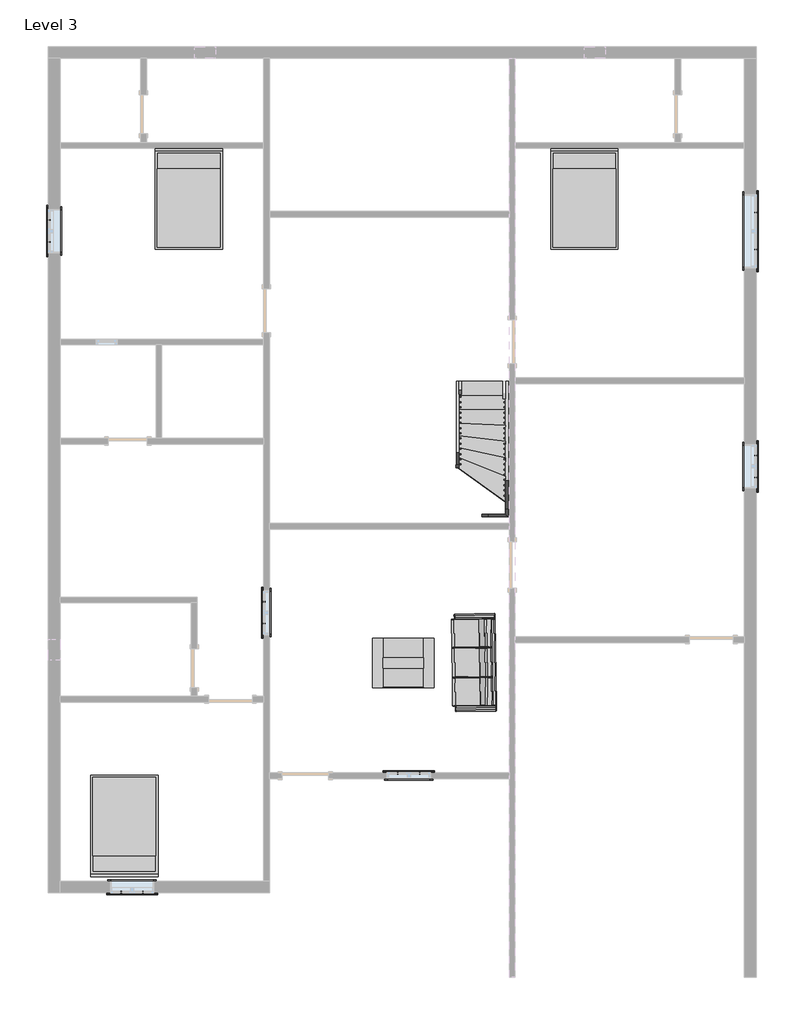
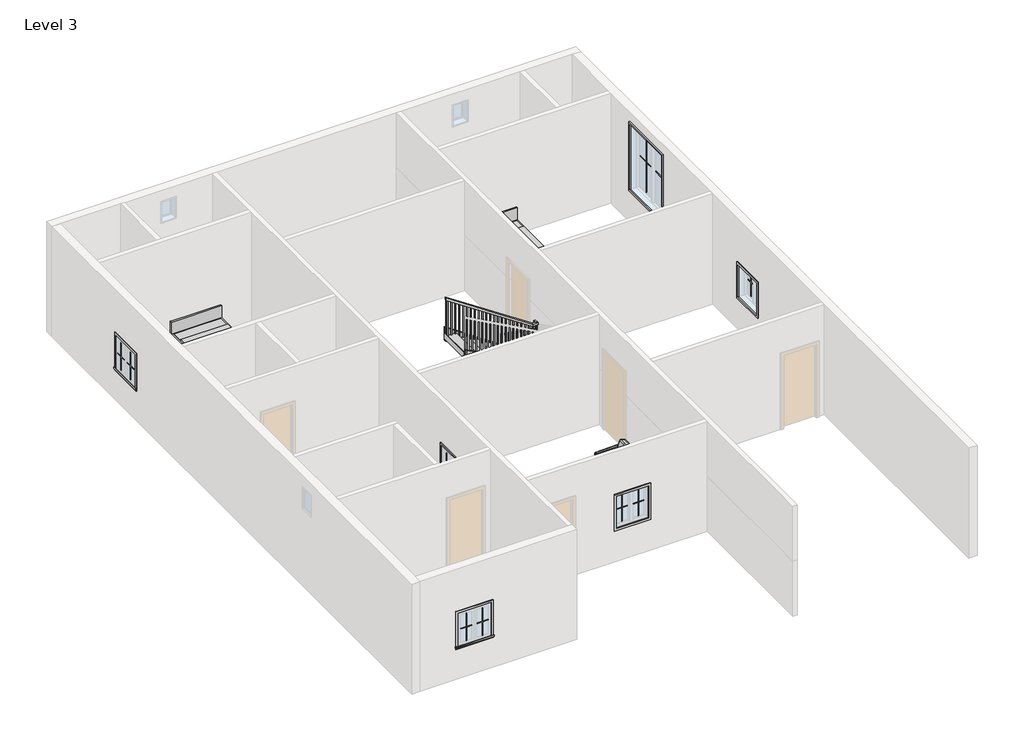
# One storey, part 3 of 3: 24 proxies, 6 members, 5 furniture elements, 1 railing, 1 stair flight.
"""IFC4 building model written with IfcOpenShell, lengths in millimetres."""

from ifc_helpers import new_model, si_unit, frame, origin, place, context, project, spatial, polyline, outline, extrude, faceted_brep, transform, mapped, element, save
from components import muntin_pattern_2x2_muntin_pattern_2x2_b3fe6957, muntin_pattern_2x2_muntin_pattern_2x2_3e0ecaf2, muntin_pattern_2x2_muntin_pattern_2x2_bff912c5, muntin_pattern_2x2_muntin_pattern_2x2_c2194282, trim_window_exterior_flat_with_sill_41619996, trim_window_exterior_flat_with_sill_e04b3088, trim_window_interior_flat_picture_frame_51c85655, trim_window_interior_flat_picture_frame_2a7685fe, furniture_2fc85b74, furniture_29a9adb8, furniture_57072a26, bed_17739_bed_17739_15c61121, wood_and_glass_coffee_table_17065_wood_and_glass_coffee_dbc724b2, stair_flight_11d19efb

model = new_model("IFC4")

# Units and contexts
model_context = context("Model", 3, world=origin())
ifc_project = project(units=[si_unit("LENGTHUNIT", "METRE", prefix="MILLI")], contexts=[model_context])

# Site, building, storey
site = spatial("IfcSite", under=ifc_project)
building = spatial("IfcBuilding", under=site)
storey = spatial("IfcBuildingStorey", under=building, Name="Level 3", Elevation=3200.4)

# Proxies
placement = place(None, origin())
muntin_pattern_2x2_muntin_pattern_2x2_shape = muntin_pattern_2x2_muntin_pattern_2x2_b3fe6957(model_context)
element("IfcBuildingElementProxy", 1, Name="Muntin Pattern_2x2 : Muntin Pattern_2x2", ObjectType="Muntin Pattern_2x2 : Muntin Pattern_2x2", at=placement, inside=storey, context=model_context, shape_type="MappedRepresentation", body=[
    mapped(muntin_pattern_2x2_muntin_pattern_2x2_shape, transform((-7494.1165084, 6600.4397623, 4184.65), x_axis=(0.0, 1.0, 0.0), y_axis=(-1.0, 0.0, 0.0), z_axis=(0.0, 0.0, 1.0))),
])
element("IfcBuildingElementProxy", 2, Name="Muntin Pattern_2x2 : Muntin Pattern_2x2", ObjectType="Muntin Pattern_2x2 : Muntin Pattern_2x2", at=placement, inside=storey, context=model_context, shape_type="MappedRepresentation", body=[
    mapped(muntin_pattern_2x2_muntin_pattern_2x2_shape, transform((-5651.0290084, -6136.0727377, 4184.65), x_axis=(-1.0, 0.0, 0.0), y_axis=(0.0, -1.0, 0.0), z_axis=(0.0, 0.0, 1.0))),
])
element("IfcBuildingElementProxy", 3, Name="Muntin Pattern_2x2 : Muntin Pattern_2x2", ObjectType="Muntin Pattern_2x2 : Muntin Pattern_2x2", at=placement, inside=storey, context=model_context, shape_type="MappedRepresentation", body=[
    mapped(muntin_pattern_2x2_muntin_pattern_2x2_shape, transform((-656.7540084, -3805.6227377, 4184.65), x_axis=(1.0, 0.0, 0.0), y_axis=(0.0, 1.0, 0.0), z_axis=(0.0, 0.0, 1.0))),
])
element("IfcBuildingElementProxy", 4, Name="Muntin Pattern_2x2 : Muntin Pattern_2x2", ObjectType="Muntin Pattern_2x2 : Muntin Pattern_2x2", at=placement, inside=storey, context=model_context, shape_type="MappedRepresentation", body=[
    mapped(muntin_pattern_2x2_muntin_pattern_2x2_shape, transform((6355.2334916, 2418.9647623, 4184.65), x_axis=(0.0, -1.0, 0.0), y_axis=(1.0, 0.0, 0.0), z_axis=(0.0, 0.0, 1.0))),
])
element("IfcBuildingElementProxy", 5, Name="Muntin Pattern_2x2 : Muntin Pattern_2x2", ObjectType="Muntin Pattern_2x2 : Muntin Pattern_2x2", at=placement, inside=storey, context=model_context, shape_type="MappedRepresentation", body=[
    mapped(muntin_pattern_2x2_muntin_pattern_2x2_shape, transform((-3277.7165084, -873.5102377, 4184.65), x_axis=(0.0, 1.0, 0.0), y_axis=(-1.0, 0.0, 0.0), z_axis=(0.0, 0.0, 1.0))),
])
muntin_pattern_2x2_muntin_pattern_2x2_2_shape = muntin_pattern_2x2_muntin_pattern_2x2_3e0ecaf2(model_context)
element("IfcBuildingElementProxy", 6, Name="Muntin Pattern_2x2 : Muntin Pattern_2x2", ObjectType="Muntin Pattern_2x2 : Muntin Pattern_2x2", at=placement, inside=storey, context=model_context, shape_type="MappedRepresentation", body=[
    mapped(muntin_pattern_2x2_muntin_pattern_2x2_2_shape, transform((-7494.1165084, 7029.0647623, 4184.65), x_axis=(0.0, -1.0, 0.0), y_axis=(1.0, 0.0, 0.0), z_axis=(0.0, 0.0, 1.0))),
])
element("IfcBuildingElementProxy", 7, Name="Muntin Pattern_2x2 : Muntin Pattern_2x2", ObjectType="Muntin Pattern_2x2 : Muntin Pattern_2x2", at=placement, inside=storey, context=model_context, shape_type="MappedRepresentation", body=[
    mapped(muntin_pattern_2x2_muntin_pattern_2x2_2_shape, transform((-6079.6540084, -6136.0727377, 4184.65), x_axis=(1.0, 0.0, 0.0), y_axis=(0.0, 1.0, 0.0), z_axis=(0.0, 0.0, 1.0))),
])
element("IfcBuildingElementProxy", 8, Name="Muntin Pattern_2x2 : Muntin Pattern_2x2", ObjectType="Muntin Pattern_2x2 : Muntin Pattern_2x2", at=placement, inside=storey, context=model_context, shape_type="MappedRepresentation", body=[
    mapped(muntin_pattern_2x2_muntin_pattern_2x2_2_shape, transform((-228.1290084, -3805.6227377, 4184.65), x_axis=(-1.0, 0.0, 0.0), y_axis=(0.0, -1.0, 0.0), z_axis=(0.0, 0.0, 1.0))),
])
element("IfcBuildingElementProxy", 9, Name="Muntin Pattern_2x2 : Muntin Pattern_2x2", ObjectType="Muntin Pattern_2x2 : Muntin Pattern_2x2", at=placement, inside=storey, context=model_context, shape_type="MappedRepresentation", body=[
    mapped(muntin_pattern_2x2_muntin_pattern_2x2_2_shape, transform((6355.2334916, 1990.3397623, 4184.65), x_axis=(0.0, 1.0, 0.0), y_axis=(-1.0, 0.0, 0.0), z_axis=(0.0, 0.0, 1.0))),
])
element("IfcBuildingElementProxy", 10, Name="Muntin Pattern_2x2 : Muntin Pattern_2x2", ObjectType="Muntin Pattern_2x2 : Muntin Pattern_2x2", at=placement, inside=storey, context=model_context, shape_type="MappedRepresentation", body=[
    mapped(muntin_pattern_2x2_muntin_pattern_2x2_2_shape, transform((-3277.7165084, -444.8852377, 4184.65), x_axis=(0.0, -1.0, 0.0), y_axis=(1.0, 0.0, 0.0), z_axis=(0.0, 0.0, 1.0))),
])
muntin_pattern_2x2_muntin_pattern_2x2_3_shape = muntin_pattern_2x2_muntin_pattern_2x2_bff912c5(model_context)
element("IfcBuildingElementProxy", 11, Name="Muntin Pattern_2x2 : Muntin Pattern_2x2", ObjectType="Muntin Pattern_2x2 : Muntin Pattern_2x2", at=placement, inside=storey, context=model_context, shape_type="MappedRepresentation", body=[
    mapped(muntin_pattern_2x2_muntin_pattern_2x2_3_shape, transform((6355.2334916, 7175.1147623, 4184.65), x_axis=(0.0, -1.0, 0.0), y_axis=(1.0, 0.0, 0.0), z_axis=(0.0, 0.0, 1.0))),
])
muntin_pattern_2x2_muntin_pattern_2x2_4_shape = muntin_pattern_2x2_muntin_pattern_2x2_c2194282(model_context)
element("IfcBuildingElementProxy", 12, Name="Muntin Pattern_2x2 : Muntin Pattern_2x2", ObjectType="Muntin Pattern_2x2 : Muntin Pattern_2x2", at=placement, inside=storey, context=model_context, shape_type="MappedRepresentation", body=[
    mapped(muntin_pattern_2x2_muntin_pattern_2x2_4_shape, transform((6355.2334916, 6454.3897623, 4184.65), x_axis=(0.0, 1.0, 0.0), y_axis=(-1.0, 0.0, 0.0), z_axis=(0.0, 0.0, 1.0))),
])
trim_window_exterior_flat_with_sill_shape = trim_window_exterior_flat_with_sill_41619996(model_context)
element("IfcBuildingElementProxy", 13, Name="Trim-Window-Exterior-Flat : with Sill", ObjectType="Trim-Window-Exterior-Flat : with Sill", at=placement, inside=storey, context=model_context, shape_type="MappedRepresentation", body=[
    mapped(trim_window_exterior_flat_with_sill_shape, transform((-7503.6415084, 6814.7522623, 5029.2), x_axis=(0.0, -1.0, 0.0), y_axis=(0.0, 0.0, 1.0), z_axis=(-1.0, 0.0, 0.0))),
])
element("IfcBuildingElementProxy", 14, Name="Trim-Window-Exterior-Flat : with Sill", ObjectType="Trim-Window-Exterior-Flat : with Sill", at=placement, inside=storey, context=model_context, shape_type="MappedRepresentation", body=[
    mapped(trim_window_exterior_flat_with_sill_shape, transform((-5865.3415084, -6145.5977377, 5029.2), x_axis=(1.0, 0.0, 0.0), y_axis=(0.0, 0.0, 1.0), z_axis=(0.0, -1.0, 0.0))),
])
element("IfcBuildingElementProxy", 15, Name="Trim-Window-Exterior-Flat : with Sill", ObjectType="Trim-Window-Exterior-Flat : with Sill", at=placement, inside=storey, context=model_context, shape_type="MappedRepresentation", body=[
    mapped(trim_window_exterior_flat_with_sill_shape, transform((-442.4415084, -3796.0977377, 5029.2), x_axis=(-1.0, 0.0, 0.0), y_axis=(0.0, 0.0, 1.0), z_axis=(0.0, 1.0, 0.0))),
])
element("IfcBuildingElementProxy", 16, Name="Trim-Window-Exterior-Flat : with Sill", ObjectType="Trim-Window-Exterior-Flat : with Sill", at=placement, inside=storey, context=model_context, shape_type="MappedRepresentation", body=[
    mapped(trim_window_exterior_flat_with_sill_shape, transform((6364.7584916, 2204.6522623, 5029.2), x_axis=(0.0, 1.0, 0.0), y_axis=(0.0, 0.0, 1.0), z_axis=(1.0, 0.0, 0.0))),
])
element("IfcBuildingElementProxy", 17, Name="Trim-Window-Exterior-Flat : with Sill", ObjectType="Trim-Window-Exterior-Flat : with Sill", at=placement, inside=storey, context=model_context, shape_type="MappedRepresentation", body=[
    mapped(trim_window_exterior_flat_with_sill_shape, transform((-3287.2415084, -659.1977377, 5029.2), x_axis=(0.0, -1.0, 0.0), y_axis=(0.0, 0.0, 1.0), z_axis=(-1.0, 0.0, 0.0))),
])
trim_window_exterior_flat_with_sill_2_shape = trim_window_exterior_flat_with_sill_e04b3088(model_context)
element("IfcBuildingElementProxy", 18, Name="Trim-Window-Exterior-Flat : with Sill", ObjectType="Trim-Window-Exterior-Flat : with Sill", at=placement, inside=storey, context=model_context, shape_type="MappedRepresentation", body=[
    mapped(trim_window_exterior_flat_with_sill_2_shape, transform((6364.7584916, 6814.7522623, 5943.6), x_axis=(0.0, 1.0, 0.0), y_axis=(0.0, 0.0, 1.0), z_axis=(1.0, 0.0, 0.0))),
])
trim_window_interior_flat_picture_frame_shape = trim_window_interior_flat_picture_frame_51c85655(model_context)
element("IfcBuildingElementProxy", 19, Name="Trim-Window-Interior-Flat : Picture Frame", ObjectType="Trim-Window-Interior-Flat : Picture Frame", at=placement, inside=storey, context=model_context, shape_type="MappedRepresentation", body=[
    mapped(trim_window_interior_flat_picture_frame_shape, transform((-7275.0415084, 6814.7522623, 5029.2), x_axis=(0.0, 1.0, 0.0), y_axis=(0.0, 0.0, 1.0), z_axis=(1.0, 0.0, 0.0))),
])
element("IfcBuildingElementProxy", 20, Name="Trim-Window-Interior-Flat : Picture Frame", ObjectType="Trim-Window-Interior-Flat : Picture Frame", at=placement, inside=storey, context=model_context, shape_type="MappedRepresentation", body=[
    mapped(trim_window_interior_flat_picture_frame_shape, transform((-5865.3415084, -5916.9977377, 5029.2), x_axis=(-1.0, 0.0, 0.0), y_axis=(0.0, 0.0, 1.0), z_axis=(0.0, 1.0, 0.0))),
])
element("IfcBuildingElementProxy", 21, Name="Trim-Window-Interior-Flat : Picture Frame", ObjectType="Trim-Window-Interior-Flat : Picture Frame", at=placement, inside=storey, context=model_context, shape_type="MappedRepresentation", body=[
    mapped(trim_window_interior_flat_picture_frame_shape, transform((-442.4415084, -3910.3977377, 5029.2), x_axis=(1.0, 0.0, 0.0), y_axis=(0.0, 0.0, 1.0), z_axis=(0.0, -1.0, 0.0))),
])
element("IfcBuildingElementProxy", 22, Name="Trim-Window-Interior-Flat : Picture Frame", ObjectType="Trim-Window-Interior-Flat : Picture Frame", at=placement, inside=storey, context=model_context, shape_type="MappedRepresentation", body=[
    mapped(trim_window_interior_flat_picture_frame_shape, transform((6136.1584916, 2204.6522623, 5029.2), x_axis=(0.0, -1.0, 0.0), y_axis=(0.0, 0.0, 1.0), z_axis=(-1.0, 0.0, 0.0))),
])
element("IfcBuildingElementProxy", 23, Name="Trim-Window-Interior-Flat : Picture Frame", ObjectType="Trim-Window-Interior-Flat : Picture Frame", at=placement, inside=storey, context=model_context, shape_type="MappedRepresentation", body=[
    mapped(trim_window_interior_flat_picture_frame_shape, transform((-3172.9415084, -659.1977377, 5029.2), x_axis=(0.0, 1.0, 0.0), y_axis=(0.0, 0.0, 1.0), z_axis=(1.0, 0.0, 0.0))),
])
trim_window_interior_flat_picture_frame_2_shape = trim_window_interior_flat_picture_frame_2a7685fe(model_context)
element("IfcBuildingElementProxy", 24, Name="Trim-Window-Interior-Flat : Picture Frame", ObjectType="Trim-Window-Interior-Flat : Picture Frame", at=placement, inside=storey, context=model_context, shape_type="MappedRepresentation", body=[
    mapped(trim_window_interior_flat_picture_frame_2_shape, transform((6136.1584916, 6814.7522623, 5943.6), x_axis=(0.0, -1.0, 0.0), y_axis=(0.0, 0.0, 1.0), z_axis=(-1.0, 0.0, 0.0))),
])

# Furniture
furniture_shape = furniture_2fc85b74(model_context)
furniture_2_shape = furniture_29a9adb8(model_context)
furniture_3_shape = furniture_57072a26(model_context)
element("IfcFurniture", 25, at=placement, inside=storey, context=model_context, shape_type="MappedRepresentation", body=[
    mapped(furniture_shape, transform((460.7695276, -1640.1238257, 3200.4), x_axis=(0.014042050983927294, -0.9999014055416489, 0.0), y_axis=(0.9999014055416489, 0.014042050983927294, 0.0), z_axis=(0.0, 0.0, 1.0))),
    mapped(furniture_2_shape, transform((460.7695276, -1640.1238257, 3200.4), x_axis=(0.014042050983927294, -0.9999014055416489, 0.0), y_axis=(0.9999014055416489, 0.014042050983927294, 0.0), z_axis=(0.0, 0.0, 1.0))),
    mapped(furniture_3_shape, transform((460.7695276, -1640.1238257, 3200.4), x_axis=(0.014042050983927294, -0.9999014055416489, 0.0), y_axis=(0.9999014055416489, 0.014042050983927294, 0.0), z_axis=(0.0, 0.0, 1.0))),
])
bed_17739_bed_17739_shape = bed_17739_bed_17739_15c61121(model_context)
element("IfcFurniture", 26, ObjectType="Bed_17739 : Bed_17739", at=placement, inside=storey, context=model_context, shape_type="MappedRepresentation", body=[
    mapped(bed_17739_bed_17739_shape, transform((-4754.0915084, 7424.3522623, 3200.4), x_axis=(1.0, 0.0, 0.0), y_axis=(0.0, 1.0, 0.0), z_axis=(0.0, 0.0, 1.0))),
])
element("IfcFurniture", 27, ObjectType="Bed_17739 : Bed_17739", at=placement, inside=storey, context=model_context, shape_type="MappedRepresentation", body=[
    mapped(bed_17739_bed_17739_shape, transform((2998.5366507, 7424.3522623, 3200.4), x_axis=(1.0, 0.0, 0.0), y_axis=(0.0, 1.0, 0.0), z_axis=(0.0, 0.0, 1.0))),
])
element("IfcFurniture", 28, ObjectType="Bed_17739 : Bed_17739", at=placement, inside=storey, context=model_context, shape_type="MappedRepresentation", body=[
    mapped(bed_17739_bed_17739_shape, transform((-6017.7415084, -4812.0977377, 3200.4), x_axis=(-1.0, 0.0, 0.0), y_axis=(0.0, -1.0, 0.0), z_axis=(0.0, 0.0, 1.0))),
])
wood_and_glass_coffee_table_17065_wood_and_glass_coffee_shape = wood_and_glass_coffee_table_17065_wood_and_glass_coffee_dbc724b2(model_context)
element("IfcFurniture", 29, ObjectType="Wood_and_Glass_Coffee_Table_17065 : Wood_and_Glass_Coffee_Table_17065", at=placement, inside=storey, context=model_context, shape_type="MappedRepresentation", body=[
    mapped(wood_and_glass_coffee_table_17065_wood_and_glass_coffee_shape, transform((-550.3915084, -1643.4477377, 3200.4), x_axis=(1.0, 0.0, 0.0), y_axis=(0.0, 1.0, 0.0), z_axis=(0.0, 0.0, 1.0))),
])

# Members
element("IfcMember", 30, ObjectType="Stringer - 2\" Width", at=placement, inside=storey, context=model_context, shape_type="SweptSolid", body=[
    extrude(outline(polyline([(3870.4222402, 3434.0789033), (3870.4222402, 3200.4), (3655.4968958, 3200.4), (1369.1992084, 4333.0067011), (1369.1992084, 4673.1572536), (3870.4222402, 3434.0789033)])), frame((1456.2084916, 0.0, 0.0), z_axis=(1.0, 0.0, 0.0), x_axis=(0.0, 1.0, 0.0)), (0.0, 0.0, 1.0), 50.8),
])
element("IfcMember", 31, ObjectType="Stringer - 2\" Width", at=placement, inside=storey, context=model_context, shape_type="SweptSolid", body=[
    extrude(outline(polyline([(1456.2084916, 1369.1992084), (1507.0084916, 1369.1992084), (1507.0084916, 1218.1652728), (1456.2084916, 1268.9652728), (1456.2084916, 1369.1992084)])), frame((0.0, 0.0, 4333.0067011), z_axis=(0.0, 0.0, 1.0), x_axis=(1.0, 0.0, 0.0)), (0.0, 0.0, 1.0), 340.1505525),
])
element("IfcMember", 32, ObjectType="Stringer - 2\" Width", at=placement, inside=storey, context=model_context, shape_type="SweptSolid", body=[
    extrude(outline(polyline([(1456.2084916, 1268.9652728), (1507.0084916, 1218.1652728), (1113.208453, 1218.1652728), (1113.208453, 1268.9652728), (1456.2084916, 1268.9652728)])), frame((0.0, 0.0, 4333.0067011), z_axis=(0.0, 0.0, 1.0), x_axis=(1.0, 0.0, 0.0)), (0.0, 0.0, 1.0), 340.1505525),
])
element("IfcMember", 33, ObjectType="Stringer - 2\" Width", at=placement, inside=storey, context=model_context, shape_type="SweptSolid", body=[
    extrude(outline(polyline([(3870.4222402, 3390.6545013), (3870.4222402, 3200.4), (3614.0281198, 3200.4), (2234.1652728, 4206.8313584), (2234.1652728, 4584.0921868), (3870.4222402, 3390.6545013)])), frame((491.0084916, 0.0, 0.0), z_axis=(1.0, 0.0, 0.0), x_axis=(0.0, 1.0, 0.0)), (0.0, 0.0, 1.0), 50.8),
])
element("IfcMember", 34, ObjectType="Stringer - 2\" Width", at=placement, inside=storey, context=model_context, shape_type="SweptSolid", body=[
    extrude(outline(polyline([(4358.5835681, 541.8084916), (4726.3965617, 541.8084916), (6317.3897736, -1813.7050583), (5949.57678, -1813.7050583), (4358.5835681, 541.8084916)])), frame((0.0, 2183.3652728, 0.0), z_axis=(0.0, 1.0, 0.0), x_axis=(0.0, 0.0, 1.0)), (0.0, 0.0, 1.0), 50.8),
])
element("IfcMember", 35, ObjectType="Stringer - 2\" Width", at=placement, inside=storey, context=model_context, shape_type="SweptSolid", body=[
    extrude(outline(polyline([(4333.0067011, 1113.208453), (4673.1572536, 1113.208453), (6264.3877281, -1813.7050583), (5924.2371756, -1813.7050583), (4333.0067011, 1113.208453)])), frame((0.0, 1218.1652728, 0.0), z_axis=(0.0, 1.0, 0.0), x_axis=(0.0, 0.0, 1.0)), (0.0, 0.0, 1.0), 50.8),
])

# Railing
element("IfcRailing", 36, ObjectType="Handrail - Rectangular", at=placement, inside=storey, context=model_context, shape_type="SolidModel", body=[
    faceted_brep([(592.6084916, 3870.4222402, 4284.1333333), (592.6084916, 3870.4222402, 4221.8674881), (541.8084916, 3870.4222402, 4221.8674881), (541.8084916, 3870.4222402, 4284.1333333), (592.6084916, 2259.5652728, 5425.8596781), (592.6084916, 2208.7652728, 5399.5993253), (541.8084916, 2208.7652728, 5399.5993253), (541.8084916, 2259.5652728, 5425.8596781), (592.6084916, 2259.5652728, 5642.6092282), (592.6084916, 2208.7652728, 5591.8092282), (541.8084916, 2208.7652728, 5591.8092282), (541.8084916, 2259.5652728, 5642.6092282), (592.6084916, 2132.5652728, 5642.6092282), (592.6084916, 2132.5652728, 5591.8092282), (541.8084916, 2183.3652728, 5591.8092282), (541.8084916, 2183.3652728, 5642.6092282), (465.6084916, 2132.5652728, 5642.6092282), (450.2220288, 2132.5652728, 5591.8092282), (450.2220288, 2183.3652728, 5591.8092282), (465.6084916, 2183.3652728, 5642.6092282), (-1813.7050583, 2132.5652728, 7162.8), (-1813.7050583, 2183.3652728, 7162.8), (-1813.7050583, 2183.3652728, 7101.7379811), (-1813.7050583, 2132.5652728, 7101.7379811)], [[[0, 1, 2, 3]], [[1, 0, 4, 5]], [[2, 1, 5, 6]], [[3, 2, 6, 7]], [[0, 3, 7, 4]], [[5, 4, 8, 9]], [[6, 5, 9, 10]], [[7, 6, 10, 11]], [[4, 7, 11, 8]], [[9, 8, 12, 13]], [[10, 9, 13, 14]], [[11, 10, 14, 15]], [[8, 11, 15, 12]], [[13, 12, 16, 17]], [[14, 13, 17, 18]], [[15, 14, 18, 19]], [[12, 15, 19, 16]], [[20, 21, 22, 23]], [[17, 16, 20, 23]], [[18, 17, 23, 22]], [[19, 18, 22, 21]], [[16, 19, 21, 20]]]),
    extrude(outline(polyline([(7065.9636891, -1760.0665084), (7078.6691083, -1779.1165084), (6079.0666667, -1779.1165084), (6079.0666667, -1760.0665084), (7065.9636891, -1760.0665084)])), frame((0.0, 2148.4402728, 0.0), z_axis=(0.0, 1.0, 0.0), x_axis=(0.0, 0.0, 1.0)), (0.0, 0.0, 1.0), 19.05),
    extrude(outline(polyline([(6998.2014532, -1658.4665084), (7010.9068724, -1677.5165084), (6079.0666667, -1677.5165084), (6079.0666667, -1658.4665084), (6998.2014532, -1658.4665084)])), frame((0.0, 2148.4402728, 0.0), z_axis=(0.0, 1.0, 0.0), x_axis=(0.0, 0.0, 1.0)), (0.0, 0.0, 1.0), 19.05),
    extrude(outline(polyline([(6930.4392173, -1556.8665084), (6943.1446365, -1575.9165084), (6079.0666667, -1575.9165084), (6079.0666667, -1556.8665084), (6930.4392173, -1556.8665084)])), frame((0.0, 2148.4402728, 0.0), z_axis=(0.0, 1.0, 0.0), x_axis=(0.0, 0.0, 1.0)), (0.0, 0.0, 1.0), 19.05),
    extrude(outline(polyline([(6862.5324687, -1455.2665084), (6875.2378879, -1474.3165084), (5909.7333333, -1474.3165084), (5909.7333333, -1455.2665084), (6862.5324687, -1455.2665084)])), frame((0.0, 2148.4402728, 0.0), z_axis=(0.0, 1.0, 0.0), x_axis=(0.0, 0.0, 1.0)), (0.0, 0.0, 1.0), 19.05),
    extrude(outline(polyline([(6794.7702328, -1353.6665084), (6807.475652, -1372.7165084), (5909.7333333, -1372.7165084), (5909.7333333, -1353.6665084), (6794.7702328, -1353.6665084)])), frame((0.0, 2148.4402728, 0.0), z_axis=(0.0, 1.0, 0.0), x_axis=(0.0, 0.0, 1.0)), (0.0, 0.0, 1.0), 19.05),
    extrude(outline(polyline([(6727.0079969, -1252.0665084), (6739.7134161, -1271.1165084), (5909.7333333, -1271.1165084), (5909.7333333, -1252.0665084), (6727.0079969, -1252.0665084)])), frame((0.0, 2148.4402728, 0.0), z_axis=(0.0, 1.0, 0.0), x_axis=(0.0, 0.0, 1.0)), (0.0, 0.0, 1.0), 19.05),
    extrude(outline(polyline([(6659.245761, -1150.4665084), (6671.9511802, -1169.5165084), (5740.4, -1169.5165084), (5740.4, -1150.4665084), (6659.245761, -1150.4665084)])), frame((0.0, 2148.4402728, 0.0), z_axis=(0.0, 1.0, 0.0), x_axis=(0.0, 0.0, 1.0)), (0.0, 0.0, 1.0), 19.05),
    extrude(outline(polyline([(6591.4835251, -1048.8665084), (6604.1889444, -1067.9165084), (5740.4, -1067.9165084), (5740.4, -1048.8665084), (6591.4835251, -1048.8665084)])), frame((0.0, 2148.4402728, 0.0), z_axis=(0.0, 1.0, 0.0), x_axis=(0.0, 0.0, 1.0)), (0.0, 0.0, 1.0), 19.05),
    extrude(outline(polyline([(6523.865802, -947.2665084), (6536.5712212, -966.3165084), (5571.0666667, -966.3165084), (5571.0666667, -947.2665084), (6523.865802, -947.2665084)])), frame((0.0, 2148.4402728, 0.0), z_axis=(0.0, 1.0, 0.0), x_axis=(0.0, 0.0, 1.0)), (0.0, 0.0, 1.0), 19.05),
    extrude(outline(polyline([(6456.1035661, -845.6665084), (6468.8089853, -864.7165084), (5571.0666667, -864.7165084), (5571.0666667, -845.6665084), (6456.1035661, -845.6665084)])), frame((0.0, 2148.4402728, 0.0), z_axis=(0.0, 1.0, 0.0), x_axis=(0.0, 0.0, 1.0)), (0.0, 0.0, 1.0), 19.05),
    extrude(outline(polyline([(6388.3413302, -744.0665084), (6401.0467495, -763.1165084), (5571.0666667, -763.1165084), (5571.0666667, -744.0665084), (6388.3413302, -744.0665084)])), frame((0.0, 2148.4402728, 0.0), z_axis=(0.0, 1.0, 0.0), x_axis=(0.0, 0.0, 1.0)), (0.0, 0.0, 1.0), 19.05),
    extrude(outline(polyline([(6320.5790943, -642.4665084), (6333.2845136, -661.5165084), (5401.7333333, -661.5165084), (5401.7333333, -642.4665084), (6320.5790943, -642.4665084)])), frame((0.0, 2148.4402728, 0.0), z_axis=(0.0, 1.0, 0.0), x_axis=(0.0, 0.0, 1.0)), (0.0, 0.0, 1.0), 19.05),
    extrude(outline(polyline([(6252.8168585, -540.8665084), (6265.5222777, -559.9165084), (5401.7333333, -559.9165084), (5401.7333333, -540.8665084), (6252.8168585, -540.8665084)])), frame((0.0, 2148.4402728, 0.0), z_axis=(0.0, 1.0, 0.0), x_axis=(0.0, 0.0, 1.0)), (0.0, 0.0, 1.0), 19.05),
    extrude(outline(polyline([(6184.9101098, -439.2665084), (6197.6155291, -458.3165084), (5401.7333333, -458.3165084), (5401.7333333, -439.2665084), (6184.9101098, -439.2665084)])), frame((0.0, 2148.4402728, 0.0), z_axis=(0.0, 1.0, 0.0), x_axis=(0.0, 0.0, 1.0)), (0.0, 0.0, 1.0), 19.05),
    extrude(outline(polyline([(6117.1478739, -337.6665084), (6129.8532932, -356.7165084), (5232.4, -356.7165084), (5232.4, -337.6665084), (6117.1478739, -337.6665084)])), frame((0.0, 2148.4402728, 0.0), z_axis=(0.0, 1.0, 0.0), x_axis=(0.0, 0.0, 1.0)), (0.0, 0.0, 1.0), 19.05),
    extrude(outline(polyline([(6049.3856381, -236.0665084), (6062.0910573, -255.1165084), (5232.4, -255.1165084), (5232.4, -236.0665084), (6049.3856381, -236.0665084)])), frame((0.0, 2148.4402728, 0.0), z_axis=(0.0, 1.0, 0.0), x_axis=(0.0, 0.0, 1.0)), (0.0, 0.0, 1.0), 19.05),
    extrude(outline(polyline([(5981.6234022, -134.4665084), (5994.3288214, -153.5165084), (5063.0666667, -153.5165084), (5063.0666667, -134.4665084), (5981.6234022, -134.4665084)])), frame((0.0, 2148.4402728, 0.0), z_axis=(0.0, 1.0, 0.0), x_axis=(0.0, 0.0, 1.0)), (0.0, 0.0, 1.0), 19.05),
    extrude(outline(polyline([(5913.8611663, -32.8665084), (5926.5665855, -51.9165084), (5063.0666667, -51.9165084), (5063.0666667, -32.8665084), (5913.8611663, -32.8665084)])), frame((0.0, 2148.4402728, 0.0), z_axis=(0.0, 1.0, 0.0), x_axis=(0.0, 0.0, 1.0)), (0.0, 0.0, 1.0), 19.05),
    extrude(outline(polyline([(5846.2434432, 68.7334916), (5858.9488624, 49.6834916), (5063.0666667, 49.6834916), (5063.0666667, 68.7334916), (5846.2434432, 68.7334916)])), frame((0.0, 2148.4402728, 0.0), z_axis=(0.0, 1.0, 0.0), x_axis=(0.0, 0.0, 1.0)), (0.0, 0.0, 1.0), 19.05),
    extrude(outline(polyline([(5778.4812073, 170.3334916), (5791.1866265, 151.2834916), (4893.7333333, 151.2834916), (4893.7333333, 170.3334916), (5778.4812073, 170.3334916)])), frame((0.0, 2148.4402728, 0.0), z_axis=(0.0, 1.0, 0.0), x_axis=(0.0, 0.0, 1.0)), (0.0, 0.0, 1.0), 19.05),
    extrude(outline(polyline([(5710.7189714, 271.9334916), (5723.4243906, 252.8834916), (4893.7333333, 252.8834916), (4893.7333333, 271.9334916), (5710.7189714, 271.9334916)])), frame((0.0, 2148.4402728, 0.0), z_axis=(0.0, 1.0, 0.0), x_axis=(0.0, 0.0, 1.0)), (0.0, 0.0, 1.0), 19.05),
    extrude(outline(polyline([(5642.9567355, 373.5334916), (5655.6621547, 354.4834916), (4724.4, 354.4834916), (4724.4, 373.5334916), (5642.9567355, 373.5334916)])), frame((0.0, 2148.4402728, 0.0), z_axis=(0.0, 1.0, 0.0), x_axis=(0.0, 0.0, 1.0)), (0.0, 0.0, 1.0), 19.05),
    extrude(outline(polyline([(5575.1944996, 475.1334916), (5587.8999189, 456.0834916), (4724.4, 456.0834916), (4724.4, 475.1334916), (5575.1944996, 475.1334916)])), frame((0.0, 2148.4402728, 0.0), z_axis=(0.0, 1.0, 0.0), x_axis=(0.0, 0.0, 1.0)), (0.0, 0.0, 1.0), 19.05),
    extrude(outline(polyline([(557.6834916, 2254.3472402), (576.7334916, 2254.3472402), (576.7334916, 2235.2972402), (557.6834916, 2235.2972402), (557.6834916, 2254.3472402)])), frame((0.0, 0.0, 4385.7333333), z_axis=(0.0, 0.0, 1.0), x_axis=(1.0, 0.0, 0.0)), (0.0, 0.0, 1.0), 1206.0758948),
    extrude(outline(polyline([(2336.8972402, 5308.7832902), (2355.9472402, 5295.2812306), (2355.9472402, 4385.7333333), (2336.8972402, 4385.7333333), (2336.8972402, 5308.7832902)])), frame((557.6834916, 0.0, 0.0), z_axis=(1.0, 0.0, 0.0), x_axis=(0.0, 1.0, 0.0)), (0.0, 0.0, 1.0), 19.05),
    extrude(outline(polyline([(2438.4972402, 5236.7723054), (2457.5472402, 5223.2702458), (2457.5472402, 4216.4), (2438.4972402, 4216.4), (2438.4972402, 5236.7723054)])), frame((557.6834916, 0.0, 0.0), z_axis=(1.0, 0.0, 0.0), x_axis=(0.0, 1.0, 0.0)), (0.0, 0.0, 1.0), 19.05),
    extrude(outline(polyline([(2540.0972402, 5164.7613206), (2559.1472402, 5151.2592609), (2559.1472402, 4216.4), (2540.0972402, 4216.4), (2540.0972402, 5164.7613206)])), frame((557.6834916, 0.0, 0.0), z_axis=(1.0, 0.0, 0.0), x_axis=(0.0, 1.0, 0.0)), (0.0, 0.0, 1.0), 19.05),
    extrude(outline(polyline([(2641.6972402, 5092.7503358), (2660.7472402, 5079.2482761), (2660.7472402, 4047.0666667), (2641.6972402, 4047.0666667), (2641.6972402, 5092.7503358)])), frame((557.6834916, 0.0, 0.0), z_axis=(1.0, 0.0, 0.0), x_axis=(0.0, 1.0, 0.0)), (0.0, 0.0, 1.0), 19.05),
    extrude(outline(polyline([(2743.2972402, 5020.739351), (2762.3472402, 5007.2372913), (2762.3472402, 4047.0666667), (2743.2972402, 4047.0666667), (2743.2972402, 5020.739351)])), frame((557.6834916, 0.0, 0.0), z_axis=(1.0, 0.0, 0.0), x_axis=(0.0, 1.0, 0.0)), (0.0, 0.0, 1.0), 19.05),
    extrude(outline(polyline([(2844.8972402, 4948.7283661), (2863.9472402, 4935.2263065), (2863.9472402, 3877.7333333), (2844.8972402, 3877.7333333), (2844.8972402, 4948.7283661)])), frame((557.6834916, 0.0, 0.0), z_axis=(1.0, 0.0, 0.0), x_axis=(0.0, 1.0, 0.0)), (0.0, 0.0, 1.0), 19.05),
    extrude(outline(polyline([(2946.4972402, 4876.7173813), (2965.5472402, 4863.2153217), (2965.5472402, 3877.7333333), (2946.4972402, 3877.7333333), (2946.4972402, 4876.7173813)])), frame((557.6834916, 0.0, 0.0), z_axis=(1.0, 0.0, 0.0), x_axis=(0.0, 1.0, 0.0)), (0.0, 0.0, 1.0), 19.05),
    extrude(outline(polyline([(3048.0972402, 4804.7063965), (3067.1472402, 4791.2043368), (3067.1472402, 3708.4), (3048.0972402, 3708.4), (3048.0972402, 4804.7063965)])), frame((557.6834916, 0.0, 0.0), z_axis=(1.0, 0.0, 0.0), x_axis=(0.0, 1.0, 0.0)), (0.0, 0.0, 1.0), 19.05),
    extrude(outline(polyline([(3149.6972402, 4732.6954117), (3168.7472402, 4719.193352), (3168.7472402, 3708.4), (3149.6972402, 3708.4), (3149.6972402, 4732.6954117)])), frame((557.6834916, 0.0, 0.0), z_axis=(1.0, 0.0, 0.0), x_axis=(0.0, 1.0, 0.0)), (0.0, 0.0, 1.0), 19.05),
    extrude(outline(polyline([(3251.2972402, 4660.6844268), (3270.3472402, 4647.1823672), (3270.3472402, 3708.4), (3251.2972402, 3708.4), (3251.2972402, 4660.6844268)])), frame((557.6834916, 0.0, 0.0), z_axis=(1.0, 0.0, 0.0), x_axis=(0.0, 1.0, 0.0)), (0.0, 0.0, 1.0), 19.05),
    extrude(outline(polyline([(3352.8972402, 4588.673442), (3371.9472402, 4575.1713824), (3371.9472402, 3539.0666667), (3352.8972402, 3539.0666667), (3352.8972402, 4588.673442)])), frame((557.6834916, 0.0, 0.0), z_axis=(1.0, 0.0, 0.0), x_axis=(0.0, 1.0, 0.0)), (0.0, 0.0, 1.0), 19.05),
    extrude(outline(polyline([(3454.4972402, 4516.6624572), (3473.5472402, 4503.1603975), (3473.5472402, 3539.0666667), (3454.4972402, 3539.0666667), (3454.4972402, 4516.6624572)])), frame((557.6834916, 0.0, 0.0), z_axis=(1.0, 0.0, 0.0), x_axis=(0.0, 1.0, 0.0)), (0.0, 0.0, 1.0), 19.05),
    extrude(outline(polyline([(3556.0972402, 4444.6514724), (3575.1472402, 4431.1494127), (3575.1472402, 3539.0666667), (3556.0972402, 3539.0666667), (3556.0972402, 4444.6514724)])), frame((557.6834916, 0.0, 0.0), z_axis=(1.0, 0.0, 0.0), x_axis=(0.0, 1.0, 0.0)), (0.0, 0.0, 1.0), 19.05),
    extrude(outline(polyline([(3657.6972402, 4372.6404876), (3676.7472402, 4359.1384279), (3676.7472402, 3369.7333333), (3657.6972402, 3369.7333333), (3657.6972402, 4372.6404876)])), frame((557.6834916, 0.0, 0.0), z_axis=(1.0, 0.0, 0.0), x_axis=(0.0, 1.0, 0.0)), (0.0, 0.0, 1.0), 19.05),
    extrude(outline(polyline([(3759.2972402, 4300.6295027), (3778.3472402, 4287.1274431), (3778.3472402, 3369.7333333), (3759.2972402, 3369.7333333), (3759.2972402, 4300.6295027)])), frame((557.6834916, 0.0, 0.0), z_axis=(1.0, 0.0, 0.0), x_axis=(0.0, 1.0, 0.0)), (0.0, 0.0, 1.0), 19.05),
    extrude(outline(polyline([(557.6834916, 2167.4902728), (576.7334916, 2167.4902728), (576.7334916, 2148.4402728), (557.6834916, 2148.4402728), (557.6834916, 2167.4902728)])), frame((0.0, 0.0, 4555.0666667), z_axis=(0.0, 0.0, 1.0), x_axis=(1.0, 0.0, 0.0)), (0.0, 0.0, 1.0), 1036.7425615),
    extrude(outline(polyline([(7089.0325619, -1794.6550583), (7101.7379811, -1813.7050583), (6079.0666667, -1813.7050583), (6079.0666667, -1794.6550583), (7089.0325619, -1794.6550583)])), frame((0.0, 2148.4402728, 0.0), z_axis=(0.0, 1.0, 0.0), x_axis=(0.0, 0.0, 1.0)), (0.0, 0.0, 1.0), 19.05),
    extrude(outline(polyline([(3851.3722402, 4235.3695477), (3870.4222402, 4221.8674881), (3870.4222402, 3369.7333333), (3851.3722402, 3369.7333333), (3851.3722402, 4235.3695477)])), frame((557.6834916, 0.0, 0.0), z_axis=(1.0, 0.0, 0.0), x_axis=(0.0, 1.0, 0.0)), (0.0, 0.0, 1.0), 19.05),
])

# Stair flight
stair_flight_shape = stair_flight_11d19efb(model_context)
element("IfcStairFlight", 37, ObjectType="2\" Tread 1\" Nosing 1/4\" Riser", at=placement, inside=storey, context=model_context, shape_type="MappedRepresentation", body=[
    mapped(stair_flight_shape, transform((0.0, 0.0, 0.0), x_axis=(1.0, 0.0, 0.0), y_axis=(0.0, 1.0, 0.0), z_axis=(0.0, 0.0, 1.0))),
])

save(model, "model.ifc")

# Revit data of these elements
# Type "Muntin Pattern_2x2 : Muntin Pattern_2x2"
#   Width [instance default] = 4' - 0"
#   Thickness = 0' - 0 1/2"
#   Height [instance default] = 4' - 0"
#   Distance = 0' - 0 3/4"
#   Interior Material [instance default] = none
#   Exterior Material [instance default] = none
#   Default Elevation = 0
# Type "Trim-Window-Exterior-Flat : with Sill"
#   Trim Width = 0' - 2 1/4"
#   Trim Thickness_Picture Frame = 0' - 1 1/4"
#   Trim Thickness_with Sill = 0' - 0 3/4"
#   Sill Thickness = 0' - 1 1/4"
#   Opening Width [instance default] = 2' - 0"
#   Opening Height [instance default] = 3' - 0"
#   Default Elevation = 4' - 0"
#   Sill = yes
#   Picture Frame = no
#   Trim Material [instance default] = none
# Type "Trim-Window-Interior-Flat : Picture Frame"
#   Trim Thickness_Picture Frame = 0' - 1 1/4"
#   Trim Width = 0' - 2 1/4"
#   Trim Thickness_with Sill = 0' - 0 3/4"
#   Sill Thickness = 0' - 1 1/4"
#   Opening Width [instance default] = 2' - 0"
#   Opening Height [instance default] = 3' - 0"
#   Default Elevation = 4' - 0"
#   Sill = no
#   Picture Frame = yes
#   Trim Material [instance default] = none
# Type
#   Width [instance] = 6' - 3.19685"
#   Default Elevation = 0
# Type "Bed_17739 : Bed_17739"
#   Default Elevation = 0
# Type "Wood_and_Glass_Coffee_Table_17065 : Wood_and_Glass_Coffee_Table_17065"
#   Coffee Table Wood Width = 0' - 7.87402"
#   Coffee Table Width = 3' - 2.17592"
#   Coffee Table Length = 3' - 11.24409"
#   Wood and Glass Coffee Table - Wood = Wood and Glass Coffee Table - Wood
#   Wood and Glass Coffee Table - Glass = Wood and Glass Coffee Table - Glass
#   Default Elevation = 0
# Type "Handrail - Rectangular"
#   Assembly Code = "C2010400"
#   built-in parameter 1008612 = 0.0416667 (stored number, unit not read)
#   built-in parameter 1008611 = 0.0416667 (stored number, unit not read)
#   built-in parameter 1008609 = 0.333333 (stored number, unit not read)
#   built-in parameter 1008604 = 0.166667 (stored number, unit not read)
#   built-in parameter 1008603 = 0.166667 (stored number, unit not read)
#   Railing Height = 3' - 0"
#   built-in parameter 1008630 = 2
#   built-in parameter 1008610 = 2
#   built-in parameter 1008618 = Baluster - Square : 3/4"
# Elements 1, 2, 3, 4, 5, 6, 7, 8, 9, 10 (IfcBuildingElementProxy, "Muntin Pattern_2x2 : Muntin Pattern_2x2")
#   Width = 0' - 11 5/8"
#   Height = 2' - 6 1/2"
#   Interior Material = Wood - Stained
#   Exterior Material = Clad - White
#   Phase Created = New Construction
#   Materials on its faces: "Clad - White", "Wood - Stained"
# Elements 11, 12 (IfcBuildingElementProxy, "Muntin Pattern_2x2 : Muntin Pattern_2x2")
#   Width = 1' - 11 1/8"
#   Height = 5' - 6 1/2"
#   Interior Material = Wood - Stained
#   Exterior Material = Clad - White
#   Phase Created = New Construction
#   Materials on its faces: "Clad - White", "Wood - Stained"
# Elements 13, 14, 15, 16, 17 (IfcBuildingElementProxy, "Trim-Window-Exterior-Flat : with Sill")
#   Opening Width = 2' - 10"
#   Opening Height = 3' - 0"
#   Trim Material = Clad - White
#   Phase Created = New Construction
#   Materials on its faces: "Clad - White"
# Element 18 (IfcBuildingElementProxy, "Trim-Window-Exterior-Flat : with Sill")
#   Opening Width = 4' - 9"
#   Opening Height = 6' - 0"
#   Trim Material = Clad - White
#   Phase Created = New Construction
#   Materials on its faces: "Clad - White"
# Elements 19, 20, 21, 22, 23 (IfcBuildingElementProxy, "Trim-Window-Interior-Flat : Picture Frame")
#   Opening Width = 2' - 10"
#   Opening Height = 3' - 0"
#   Trim Material = Wood - Stained
#   Phase Created = New Construction
#   Materials on its faces: "Wood - Stained"
# Element 24 (IfcBuildingElementProxy, "Trim-Window-Interior-Flat : Picture Frame")
#   Opening Width = 4' - 9"
#   Opening Height = 6' - 0"
#   Trim Material = Wood - Stained
#   Phase Created = New Construction
#   Materials on its faces: "Wood - Stained"
# Element 25 (IfcFurniture)
#   Width = 6' - 3.19685"
#   Phase Created = New Construction
# Elements 26, 27, 28 (IfcFurniture, "Bed_17739 : Bed_17739")
#   Phase Created = New Construction
#   Materials on its faces: "legs", "sheets", "bed frame", "Blanket"
# Element 29 (IfcFurniture, "Wood_and_Glass_Coffee_Table_17065 : Wood_and_Glass_Coffee_Table_17065")
#   Phase Created = New Construction
#   Materials on its faces: "Wood and Glass Coffee Table - Wood", "Wood and Glass Coffee Table - Glass"
# Elements 30, 31, 32, 33, 34, 35 (IfcMember, "Stringer - 2\" Width")
#   Phase Created = New Construction
# Element 36 (IfcRailing, "Handrail - Rectangular")
#   Phase Created = New Construction
# Element 37 (IfcStairFlight, "2\" Tread 1\" Nosing 1/4\" Riser")
#   Phase Created = New Construction
# Materials
#   "Wood and Glass Coffee Table - Wood": class "Generic", colour RGB 120 120 120, transparency 0, Cost = 0
#   "Wood and Glass Coffee Table - Glass": class "Generic", colour RGB 120 120 120, transparency 0, Cost = 0
#   "Clad - White": class "Wood", colour RGB 242 242 238, transparency 0, Cost = 0
#   "Wood - Stained": class "Wood", colour RGB 224 178 126, transparency 0, Cost = 0
#   "legs": colour RGB 90 73 37, transparency 0, Cost = 0
#   "sheets": colour RGB 200 195 176, transparency 0, Cost = 0
#   "bed frame": colour RGB 90 73 37, transparency 0, Cost = 0
#   "Blanket": class "System", colour RGB 59 0 1, transparency 0, Cost = 0
